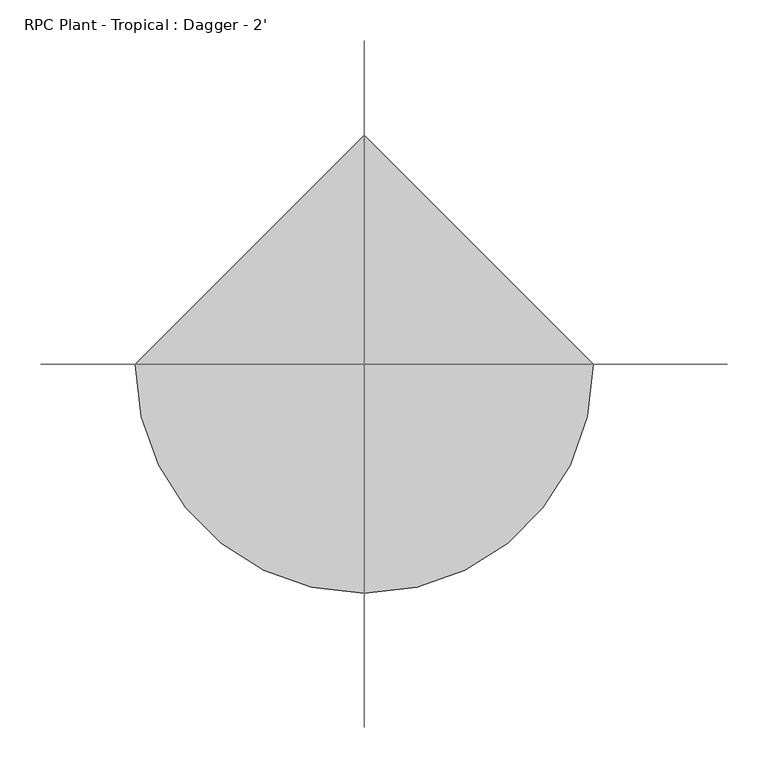
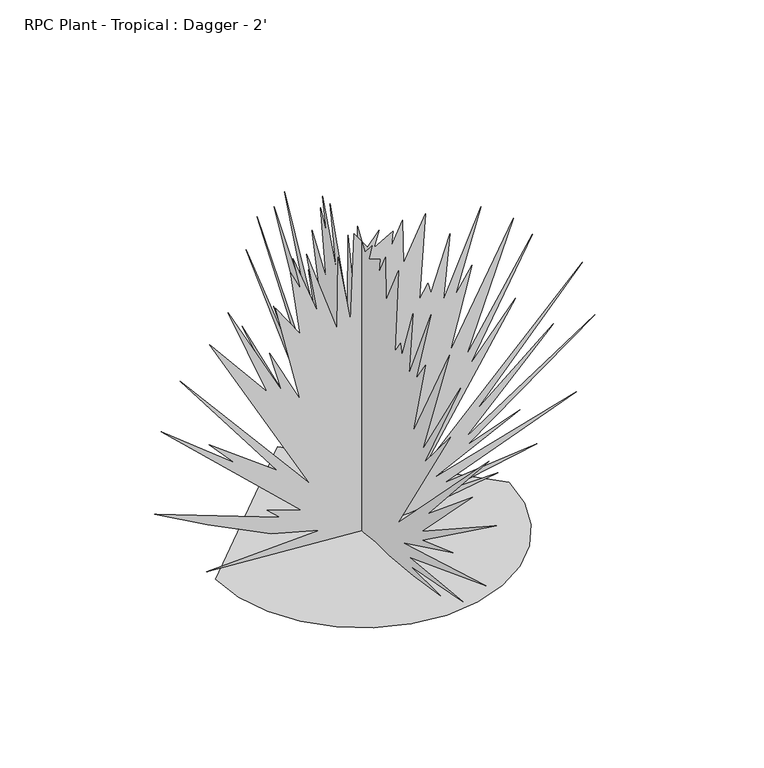
"""IFC4 building model written with IfcOpenShell, lengths in millimetres: geographic element geometry, RPC Plant - Tropical : Dagger - 2'."""

from ifc_helpers import new_model, si_unit, origin, place, context, project, spatial, triangles, source, transform, mapped, element, save


def rpc_plant_tropical_dagger_2_80c14bd7(model_context):
    return source(origin(), model_context, "Body", "Tessellation", [
        triangles([(-0.0169483, -5.816808, 0.0), (-0.0169288, 298.9836399, 21.1666745), (-0.0169413, 81.6722405, 29.6334406), (-0.0169342, 174.805482, 55.033464), (-0.0169232, 297.5713896, 117.1222841), (-0.0169138, 399.1714926, 173.5667131), (-0.0169336, 157.8723041, 83.2556831), (-0.0169307, 183.2723162, 105.8335019), (-0.016936, 116.9500744, 83.2556831), (-0.0169048, 386.4714684, 337.2563765), (-0.0169199, 245.3611499, 224.3667555), (-0.0169138, 294.7494507, 277.9879738), (-0.0169274, 163.5166906, 180.6223326), (-0.0169017, 349.7836641, 426.1564734), (-0.0169339, 101.427866, 132.6444926), (-0.0169017, 293.339762, 481.1881433), (-0.0169163, 183.2723162, 347.1344436), (-0.0169007, 258.0616646, 533.400436), (-0.0169184, 155.0501108, 340.0783336), (-0.0169121, 177.6279296, 423.3345162), (-0.0169223, 119.7722677, 309.0344436), (-0.0169075, 166.3388839, 510.8223447), (-0.0169144, 119.7722677, 443.088107), (-0.0169055, 138.1166785, 572.9127045), (-0.016909, 118.3610439, 533.400436), (-0.0169042, 132.4722829, 599.7224052), (-0.0169145, 85.9054123, 475.5442655), (-0.0169058, 107.0722617, 599.7224052), (-0.0169196, 47.8056303, 427.566162), (-0.016911, 46.3944065, 572.9127045), (-0.0169207, 22.4054592, 434.622272), (-0.0169106, 15.349867, 609.6005087), (-0.0169144, -10.050077, 572.9127045), (-0.0169141, -32.6278504, 599.7224052), (-0.0169154, -22.7501125, 567.2662831), (-0.0169164, -59.4390954, 588.4346495), (-0.0169179, -56.6168975, 560.2126802), (-0.0169166, -77.7834971, 603.9565945), (-0.0169218, -79.1947209, 516.4662226), (-0.0169192, -121.52792, 602.5443624), (-0.0169287, -110.2391378, 431.8003512), (-0.0169282, -127.17257, 458.6125955), (-0.0169297, -132.8169566, 437.4442291), (-0.0169255, -169.5057691, 544.6881918), (-0.0169325, -156.8057631, 414.8661378), (-0.0169271, -228.7723914, 578.5565824), (-0.0169337, -179.3835819, 417.6880949), (-0.0169328, -211.8392135, 465.6661983), (-0.0169399, -169.5057691, 304.8002543), (-0.0169334, -290.8607164, 533.400436), (-0.0169428, -200.550186, 286.4563522), (-0.0169383, -327.5510459, 488.2442533), (-0.0169445, -207.6057873, 265.2879677), (-0.0169435, -295.0948874, 369.7125349), (-0.0169498, -120.1169505, 88.9000696), (-0.0169494, -423.5072528, 397.9345041), (-0.016951, -218.8948329, 167.9223265), (-0.0169525, -368.473003, 292.1002301), (-0.0169526, -199.1392074, 119.9444865), (-0.0169578, -447.4950328, 282.222163), (-0.0169538, -201.9614007, 103.0113086), (-0.0169577, -303.5607224, 139.700112), (-0.0169526, -137.0501284, 59.2666313), (-0.0169642, -412.2169172, 138.2888882), (-0.0169548, -158.2169778, 42.3334534), (-0.0169644, -336.0168809, 59.2666313), (-0.0169559, -159.6279563, 25.4000212), (-0.0169619, -261.2290403, 26.811245), (-0.0169573, -170.9169838, 12.7000106), (-0.0169529, -89.0722793, 4.2333197), (-0.0169503, -43.9168869, 4.2333197), (-282.2577168, 0.0, 0.0937388), (-274.7951999, -64.6747996, 0.0937388), (-253.5445348, -124.0684354, 0.0937388), (-220.2049637, -176.4790898, 0.0937388), (-176.4790898, -220.2049637, 0.0937388), (-124.0684354, -253.5445348, 0.0937388), (-64.6747996, -274.7951999, 0.0937388), (1.23e-05, -282.2577168, 0.0937388), (64.6747996, -274.7951999, 0.0937388), (124.0684354, -253.5445348, 0.0937388), (176.4790898, -220.2049637, 0.0937388), (220.2049637, -176.4790898, 0.0937388), (253.5445348, -124.0684354, 0.0937388), (274.7951999, -64.6747996, 0.0937388), (282.2577168, 2.47e-05, 0.0937388), (-3.7e-05, 282.2577168, 0.0937388), (5.816808, 0.0169479, 0.0), (-298.9836399, 0.0169466, 21.1666745), (-81.6722405, 0.0169461, 29.6334406), (-174.8057363, 0.0169446, 55.033464), (-297.5713896, 0.0169409, 117.1222841), (-399.1714926, 0.0169375, 173.5667131), (-157.8723041, 0.016943, 83.2556831), (-183.2723162, 0.0169416, 105.8335019), (-116.9500744, 0.016943, 83.2556831), (-386.4714684, 0.0169278, 337.2563765), (-245.3611499, 0.0169345, 224.3667555), (-294.7494507, 0.0169313, 277.9879738), (-163.5166906, 0.0169371, 180.6223326), (-349.7836641, 0.0169225, 426.1564734), (-101.427866, 0.01694, 132.6444926), (-293.339762, 0.0169192, 481.1881433), (-183.2723162, 0.0169272, 347.1344436), (-258.0616646, 0.0169161, 533.400436), (-155.0501108, 0.0169277, 340.0783336), (-177.6279296, 0.0169227, 423.3345162), (-119.7722677, 0.0169295, 309.0344436), (-166.3388839, 0.0169175, 510.8223447), (-119.7722677, 0.0169215, 443.088107), (-138.1166785, 0.0169138, 572.9127045), (-118.3610439, 0.0169161, 533.400436), (-132.4722829, 0.0169121, 599.7224052), (-85.9054123, 0.0169196, 475.5442655), (-107.0722617, 0.0169121, 599.7224052), (-47.8056303, 0.0169224, 427.566162), (-46.3944065, 0.0169138, 572.9127045), (-22.4054592, 0.016922, 434.622272), (-15.3498931, 0.0169116, 609.6005087), (10.0501019, 0.0169138, 572.9127045), (32.6278504, 0.0169121, 599.7224052), (22.7501125, 0.0169141, 567.2662831), (59.4390954, 0.0169129, 588.4346495), (56.6168975, 0.0169145, 560.2126802), (77.7834971, 0.0169119, 603.9565945), (79.1947209, 0.0169171, 516.4662226), (121.52792, 0.016912, 602.5443624), (110.2391378, 0.0169222, 431.8003512), (127.17257, 0.0169206, 458.6125955), (132.8169566, 0.0169218, 437.4442291), (169.5057691, 0.0169154, 544.6881918), (156.8057631, 0.0169232, 414.8661378), (228.7723914, 0.0169134, 578.5565824), (179.3835819, 0.016923, 417.6880949), (211.8392135, 0.0169201, 465.6661983), (169.5057691, 0.0169297, 304.8002543), (290.8607164, 0.0169161, 533.400436), (200.550186, 0.0169308, 286.4563522), (327.5510459, 0.0169188, 488.2442533), (207.6057873, 0.0169321, 265.2879677), (295.0948874, 0.0169259, 369.7125349), (120.1169505, 0.0169426, 88.9000696), (423.5072528, 0.0169242, 397.9345041), (218.8948329, 0.0169379, 167.9223265), (368.473003, 0.0169305, 292.1002301), (199.1392074, 0.0169408, 119.9444865), (447.4950328, 0.0169311, 282.222163), (201.9614007, 0.0169418, 103.0113086), (303.5607224, 0.0169396, 139.700112), (137.0501284, 0.0169444, 59.2666313), (412.2169172, 0.0169397, 138.2888882), (158.2169778, 0.0169454, 42.3334534), (336.0168809, 0.0169444, 59.2666313), (159.6279563, 0.0169464, 25.4000212), (261.2290403, 0.0169463, 26.811245), (170.9169838, 0.0169471, 12.7000106), (89.0722793, 0.0169477, 4.2333197), (43.9168869, 0.0169477, 4.2333197)], [[68, 67, 69], [69, 67, 70], [64, 63, 65], [62, 61, 63], [58, 57, 59], [56, 55, 57], [57, 55, 59], [52, 51, 53], [50, 49, 51], [48, 47, 49], [46, 45, 47], [47, 45, 49], [40, 39, 41], [36, 35, 37], [34, 33, 35], [28, 27, 29], [26, 25, 27], [24, 23, 25], [22, 21, 23], [20, 19, 21], [16, 15, 17], [12, 11, 13], [10, 9, 11], [11, 9, 13], [8, 7, 9], [2, 1, 3], [66, 65, 67], [67, 65, 70], [65, 63, 70], [60, 59, 61], [61, 59, 63], [59, 55, 63], [63, 55, 70], [54, 53, 55], [53, 51, 55], [51, 49, 55], [49, 45, 55], [44, 43, 45], [45, 43, 55], [43, 42, 55], [42, 41, 55], [55, 41, 70], [41, 39, 70], [70, 39, 71], [39, 38, 71], [38, 37, 71], [37, 35, 71], [71, 35, 1], [35, 33, 1], [33, 32, 1], [18, 17, 19], [17, 15, 19], [19, 15, 21], [14, 13, 15], [13, 9, 15], [6, 5, 7], [5, 4, 7], [4, 3, 7], [7, 3, 9], [9, 3, 15], [21, 15, 23], [23, 15, 25], [25, 15, 27], [15, 3, 27], [27, 3, 29], [3, 1, 29], [29, 1, 30], [30, 1, 31], [1, 32, 31], [86, 87, 72], [85, 86, 72], [85, 72, 73], [84, 85, 73], [84, 73, 74], [84, 74, 75], [83, 84, 75], [82, 83, 75], [82, 75, 76], [82, 76, 77], [82, 77, 78], [82, 78, 79], [82, 79, 80], [82, 80, 81], [154, 155, 156], [154, 156, 157], [150, 151, 152], [148, 149, 150], [144, 145, 146], [142, 143, 144], [142, 144, 146], [138, 139, 140], [136, 137, 138], [134, 135, 136], [132, 133, 134], [132, 134, 136], [126, 127, 128], [122, 123, 124], [120, 121, 122], [114, 115, 116], [112, 113, 114], [110, 111, 112], [108, 109, 110], [106, 107, 108], [102, 103, 104], [98, 99, 100], [96, 97, 98], [96, 98, 100], [94, 95, 96], [88, 89, 90], [152, 153, 154], [152, 154, 157], [150, 152, 157], [146, 147, 148], [146, 148, 150], [142, 146, 150], [142, 150, 157], [140, 141, 142], [138, 140, 142], [136, 138, 142], [132, 136, 142], [130, 131, 132], [130, 132, 142], [129, 130, 142], [128, 129, 142], [128, 142, 157], [126, 128, 157], [126, 157, 158], [125, 126, 158], [124, 125, 158], [122, 124, 158], [122, 158, 88], [120, 122, 88], [119, 120, 88], [104, 105, 106], [102, 104, 106], [102, 106, 108], [100, 101, 102], [96, 100, 102], [92, 93, 94], [91, 92, 94], [90, 91, 94], [90, 94, 96], [90, 96, 102], [102, 108, 110], [102, 110, 112], [102, 112, 114], [90, 102, 114], [90, 114, 116], [88, 90, 116], [88, 116, 117], [88, 117, 118], [119, 88, 118]], closed=False),
    ])


if __name__ == "__main__":
    model = new_model("IFC4")
    model_context = context("Model", 3, world=origin())
    ifc_project = project(units=[si_unit("LENGTHUNIT", "METRE", prefix="MILLI")], contexts=[model_context])
    site = spatial("IfcSite", under=ifc_project)
    building = spatial("IfcBuilding", under=site)
    placement = place(None, origin())
    rpc_plant_tropical_dagger_2_shape = rpc_plant_tropical_dagger_2_80c14bd7(model_context)
    element("IfcGeographicElement", 1, ObjectType="RPC Plant - Tropical : Dagger - 2'", at=placement, inside=building, context=model_context, shape_type="MappedRepresentation", body=[
        mapped(rpc_plant_tropical_dagger_2_shape, transform((0.0, 0.0, 0.0), x_axis=(1.0, 0.0, 0.0), y_axis=(0.0, 1.0, 0.0), z_axis=(0.0, 0.0, 1.0))),
    ])
    save(model, "model.ifc")

# Revit data of these elements
# Type "RPC Plant - Tropical : Dagger - 2'"
#   built-in parameter 1005198 = "{2, 15},{39, RPC-16-G3A7-NEG0-UH6H-J000-ST1L-LVER-AU},{1, 0},{1, 0},{2, 13},{1, 8},{5, Color},{1, 0},{1, 0},{3, 0.8},{3, 0.8},{3, 0.8},{1, 8},{7, BBoxMin},{1, 0},{1, 0},{1, 0},{1, 0},{1, 0},{1, 8},{7, BBoxMax},{1, 0},{1, 0},{1, 0},{1, 0},{1, 0},{2, 11},{9, RPCTypeId},{1, 0},{1, 0},{39, RPC-16-G3A7-NEG0-UH6H-J000-ST1L-LVER-AU},{1, 6},{14, RPCPlantHeight},{1, 0},{1, 0},{1, 2},{2, 11},{7, keyword},{1, 0},{1, 0},{35, :RPCs:Plants [General]:Geometry:RPC},{2, 11},{8, category},{1, 0},{1, 0},{16, Plants [General]},{2, 11},{12, LocalizedUID},{1, 0},{1, 0},{6, Dagger},{2, 14},{6, Height},{1, 0},{1, 0},{1, 2},{1, 2},{16, Cast Reflections},{1, 0},{1, 0},{1, 0},{1, 2},{12, Cast Shadows},{1, 0},{1, 0},{1, 1},{1, 2},{9, Lock View},{1, 0},{1, 0},{1, 0},{1, 4},{5, ViewC},{1, 0},{1, 0},{1, 0},{21, assetlibrary_base.fbx},{1, 5},"
#   built-in parameter 1005195 = "RPC-16-G3A7-NEG0-UH6H-J000-ST1L-LVER-AU"
#   Type Comments = "Dagger"
#   Assembly Code = "G2050500"
#   Height = 2' - 0"
#   Default Elevation = 0
